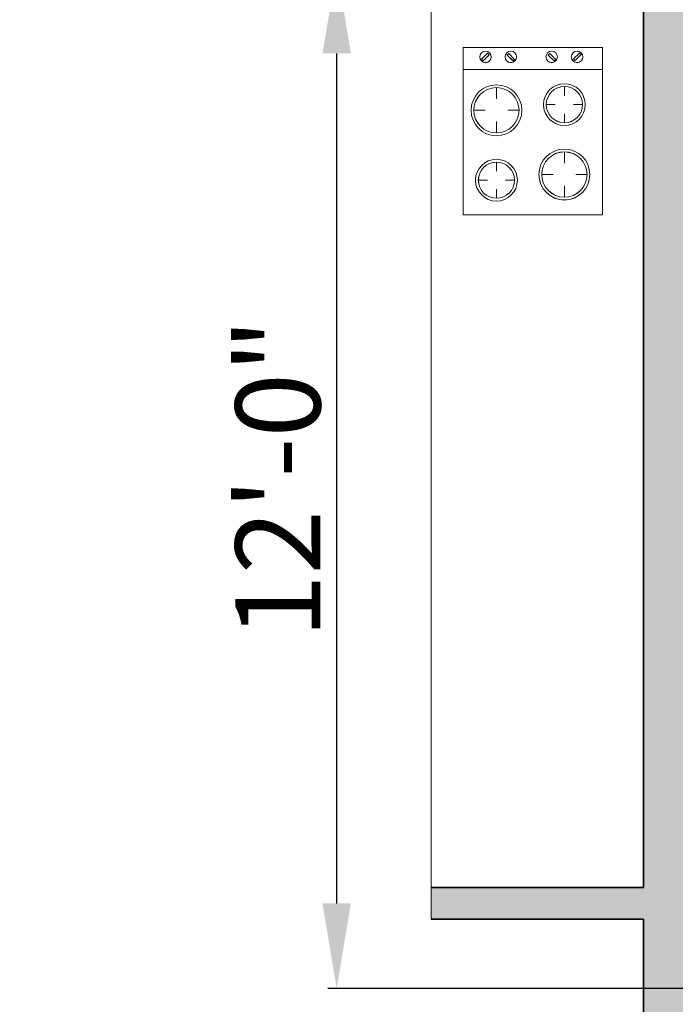
# Model space of a CAD drawing. Units: inches. Extents: x 2083 to 3317, y 1141 to 2115.
# Tile 104 of 256: x 2508 to 2600, y 1794 to 1933. Entities that reach past the tile are written whole.
import ezdxf

# ---------------------------------------------------------------- set-up
doc = ezdxf.new("R2010")
doc.units = ezdxf.units.IN
for name, color, linetype, lineweight in [('A-ANNO-DIMS', 2, 'Continuous', 18), ('A-EQPM', 8, 'Continuous', 18), ('A-FLOR-CASE', 8, 'Continuous', 18), ('A-WALL', 7, 'Continuous', 35)]:
    doc.layers.add(name, color=color, linetype=linetype, lineweight=lineweight)
doc.layers.add('A-WALL-PATT', color=251, linetype='Continuous', lineweight=13, true_color=0x636466)
doc.styles.get("Standard").update_dxf_attribs({"font": 'arial.ttf'})
doc.dimstyles.new('ISO-25', dxfattribs={"dimtxt": 12, "dimasz": 12, "dimexe": 1.25, "dimexo": 0.625, "dimtad": 1, "dimlunit": 3, "dimtxsty": 'Standard', "dimcen": 2.5, "dimadec": 0, "dimazin": 0, "dimtfac": 1, "dimtmove": 0, "dimatfit": 3, "dimfxl": 1, "dimarcsym": 0})

# ---------------------------------------------------------------- blocks, each defined once
blk = doc.blocks.new('A$C16A60262')
at = {"linetype": 'ByBlock'}
for p, q in [((0, 600), (0, 0)), ((487.7, 600), (0, 600)), ((0, 600), (500, 600)), ((0, 600), (500, 600)), ((500, 600), (500, 0)), ((500, 600), (500, 0)), ((500, 520.4), (0, 520.4)), ((363.3, 459.6), (363.3, 427.1)), ((119.4, 455.6), (119.4, 414.9)), ((298.2, 394.6), (330.7, 394.6)), ((428.3, 394.6), (395.8, 394.6)), ((38.1, 374.3), (78.8, 374.3)), ((200.7, 374.3), (160.1, 374.3)), ((363.3, 329.6), (363.3, 362.1)), ((119.4, 293), (119.4, 333.7)), ((363.3, 225.2), (363.3, 184.6)), ((119.4, 188.6), (119.4, 156.1)), ((282, 143.9), (322.6, 143.9)), ((444.5, 143.9), (403.9, 143.9)), ((54.4, 123.6), (86.9, 123.6)), ((184.4, 123.6), (151.9, 123.6)), ((119.4, 58.6), (119.4, 91.1)), ((363.3, 62.6), (363.3, 103.3)), ((0, 0), (500, 0))]:
    blk.add_line(p, q, dxfattribs=at)
for p, q in [((66.2, 557.5), (87.4, 578.7)), ((93.1, 573), (71.9, 551.8)), ((87.4, 578.7), (93.1, 573)), ((157.6, 572.5), (163.3, 578.1)), ((178.8, 551.2), (157.6, 572.5)), ((163.3, 578.1), (184.5, 556.9)), ((305.1, 572.5), (310.8, 578.1)), ((326.3, 551.2), (305.1, 572.5)), ((310.8, 578.1), (332, 556.9)), ((396.2, 558.5), (417.4, 579.7)), ((423.1, 574), (401.9, 552.8)), ((417.4, 579.7), (423.1, 574)), ((71.9, 551.8), (66.2, 557.5)), ((184.5, 556.9), (178.8, 551.2)), ((332, 556.9), (326.3, 551.2)), ((401.9, 552.8), (396.2, 558.5))]:
    blk.add_line(p, q)
for centre in [(80.1, 565.7), (171.2, 565.7), (317.6, 565.7), (408.7, 565.7)]:
    blk.add_circle(centre, 20.6)
for centre, radius in [((119.4, 374.3), 91.3), ((363.3, 394.6), 75), ((363.3, 394.6), 65), ((119.4, 374.3), 81.3), ((363.3, 143.9), 91.3), ((363.3, 143.9), 81.3), ((119.4, 123.6), 75), ((119.4, 123.6), 65)]:
    blk.add_circle(centre, radius, dxfattribs=at)
blk = doc.blocks.new('*D50')
at = {"layer": 'A-ANNO-DIMS', "color": 0, "lineweight": -2, "transparency": 16777216}
for p, q in [((2604.33, 1939.76), (2551.36, 1939.76)), ((2552.61, 1807.76), (2552.61, 1927.76)), ((2604.33, 1795.76), (2551.36, 1795.76))]:
    blk.add_line(p, q, dxfattribs=at)
at = {"layer": 'A-ANNO-DIMS', "color": 0, "transparency": 16777216}
for points in [[(2550.61, 1927.76), (2554.61, 1927.76), (2552.61, 1939.76)], [(2550.61, 1807.76), (2554.61, 1807.76), (2552.61, 1795.76)]]:
    blk.add_solid(points, dxfattribs=at)
at = {"layer": 'Defpoints', "color": 0, "transparency": 16777216}
for p in [(2552.61, 1939.76), (2604.96, 1939.76), (2604.96, 1795.76)]:
    blk.add_point(p, dxfattribs=at)
at = {"layer": 'A-ANNO-DIMS', "color": 0, "transparency": 16777216, "insert": (2545.86, 1867.76), "char_height": 12, "attachment_point": 5, "rotation": 90}
blk.add_mtext('12\'-0"', dxfattribs=at)

msp = doc.modelspace()

# ---------------------------------------------------------------- hatches: boundary and pattern name
at = {"layer": 'A-WALL-PATT'}
h = msp.add_hatch(color=256, dxfattribs=at)
h.dxf.hatch_style = 1
h.paths.add_polyline_path([(3126.96, 2020.761), (2748.96, 2020.761), (2604.96, 2020.761), (2226.96, 2020.761), (2226.96, 1702.761), (2466.96, 1702.761), (2466.96, 1582.761), (2418.96, 1582.761), (2418.96, 1477.761), (2226.96, 1477.761), (2226.96, 1263.261), (2544.96, 1263.261), (2544.96, 1411.761), (2604.96, 1411.761), (2685.96, 1411.761), (2685.96, 1420.761), (2604.96, 1420.761), (2604.96, 1573.761), (2604.96, 1702.761), (2604.96, 2011.761), (2748.96, 2011.761), (2748.96, 1702.761), (2862.96, 1702.761), (2862.96, 1621.761), (2871.96, 1621.761), (2871.96, 1702.761), (2883.96, 1702.761), (2883.96, 1706.939, -0.0264593), (2883.96, 1711.761), (2757.96, 1711.761), (2757.96, 1807.761), (2787.96, 1807.761), (2787.96, 1812.261), (2757.96, 1812.261), (2757.96, 2011.761), (2877.96, 2011.761), (2877.96, 1812.261), (2847.96, 1812.261), (2847.96, 1807.761), (2889.836, 1807.761), (2889.836, 1812.261), (2882.46, 1812.261), (2882.46, 2011.761), (3117.96, 2011.761), (3117.96, 1812.261), (2937.836, 1812.261), (2937.836, 1807.761), (2995.71, 1807.761), (2995.71, 1796.118), (3000.21, 1796.118), (3000.21, 1807.761), (3117.96, 1807.761), (3117.96, 1711.761), (3000.21, 1711.761), (3000.21, 1760.118), (2998.573, 1760.118, -0.020711), (2995.71, 1760.118), (2995.71, 1711.761), (2931.96, 1711.761), (2931.96, 1702.761), (3126.96, 1702.761)])
h.paths.add_polyline_path([(2471.46, 2011.761), (2471.46, 1810.011), (2462.717, 1810.011), (2462.717, 1805.511), (2505.96, 1805.511), (2505.96, 1810.011), (2475.96, 1810.011), (2475.96, 2011.761), (2595.96, 2011.761), (2595.96, 1810.011), (2565.96, 1810.011), (2565.96, 1805.511), (2595.96, 1805.511), (2595.96, 1711.761), (2235.96, 1711.761), (2235.96, 1805.511), (2353.71, 1805.511), (2353.71, 1796.054), (2358.21, 1796.054), (2358.21, 1805.511), (2414.717, 1805.511), (2414.717, 1810.011), (2235.96, 1810.011), (2235.96, 2011.761)], flags=16)
h.paths.add_polyline_path([(2270.205, 1994.61), (2270.205, 1970.61), (2246.205, 1970.61), (2246.205, 1994.61)], flags=0)
edge = h.paths.add_edge_path(flags=0)
edge.add_ellipse((2332.027, 1899.798), major_axis=(-3.043, 3.043), ratio=0.1682525, start_angle=-161.33217, end_angle=-156.30711, ccw=False)
edge.add_ellipse((2333.082, 1898.744), major_axis=(-1.055, 1.055), ratio=0.4535321, start_angle=-123.37102, end_angle=-94.15911)
edge = h.paths.add_edge_path(flags=0)
edge.add_ellipse((2332.027, 1968.876), major_axis=(3.043, 3.043), ratio=0.1682525, start_angle=18.66783, end_angle=23.69289)
edge.add_spline(control_points=[(2332.926, 1970.691), (2332.227, 1970.336), (2330.894, 1969.659), (2328.413, 1970.932), (2327.204, 1967.749), (2324.71, 1969.956), (2322.533, 1967.012), (2320.013, 1971.296), (2317.68, 1968.158), (2316.041, 1967.102), (2315.427, 1966.81)], knot_values=[0, 0, 0, 0, 2.2670587, 4.3245589, 6.6855835, 8.8786411, 11.121502, 14.300359, 17.7552837, 19.732645, 19.732645, 19.732645, 19.732645], degree=3, periodic=0)
edge.add_ellipse((2332.027, 1968.876), major_axis=(3.043, 3.043), ratio=0.1682525, start_angle=18.66783, end_angle=23.69289, ccw=False)
edge.add_ellipse((2333.082, 1969.931), major_axis=(1.055, 1.055), ratio=0.4535321, start_angle=56.62898, end_angle=85.84089, ccw=False)
edge = h.paths.add_edge_path(flags=0)
edge.add_spline(control_points=[(2296.428, 1967.988), (2293.628, 1965.336), (2287.704, 1959.727), (2299.744, 1949.996), (2294.533, 1935.669), (2290.573, 1920.604), (2293.394, 1909.974), (2296.185, 1904.967)], knot_values=[0.0991853, 0.0991853, 0.0991853, 0.0991853, 0.3453009, 0.6198217, 0.9826526, 1.3860932, 1.8105546, 1.8105546, 1.8105546, 1.8105546], degree=3, periodic=0)
edge.add_spline(control_points=[(2296.185, 1904.967), (2297.384, 1902.619), (2298.001, 1901.949), (2298.553, 1901.468)], knot_values=[0.0062457, 0.0062457, 0.0062457, 0.0062457, 0.0554759, 0.0554759, 0.0554759, 0.0554759], degree=3, periodic=0)
edge.add_spline(control_points=[(2298.553, 1901.468), (2297.259, 1900.923), (2295.225, 1900.232), (2293.06, 1900.614), (2292.101, 1900.788), (2292.09, 1900.791)], knot_values=[0.3128349, 0.3128349, 0.3128349, 0.3128349, 0.4017797, 0.4749867, 0.4759027, 0.4759027, 0.4759027, 0.4759027], degree=3, periodic=0)
edge.add_arc((2292.794, 1904.664), 3.937, 215.4209, 259.69818, ccw=False)
edge.add_spline(control_points=[(2289.585, 1902.382), (2289.477, 1902.535), (2289.368, 1902.688), (2289.261, 1902.841)], knot_values=[0.1028719, 0.1028719, 0.1028719, 0.1028719, 0.1168958, 0.1168958, 0.1168958, 0.1168958], degree=3, periodic=0)
edge.add_spline(control_points=[(2289.261, 1902.841), (2288.687, 1902.55), (2287.64, 1902.02), (2285.881, 1901.874), (2283.853, 1901.504), (2281.72, 1899.711), (2278.467, 1899.493), (2276.157, 1901.883), (2272.259, 1899.804), (2267.778, 1901.843), (2262.244, 1900.184), (2257.415, 1901.782), (2254.318, 1900.726), (2253.178, 1900.337)], knot_values=[0, 0, 0, 0, 1.9079767, 3.4771759, 5.261074, 7.9728515, 11.6802485, 13.7179214, 16.9395917, 22.789562, 27.5025027, 33.5952153, 37.1456181, 37.1456181, 37.1456181, 37.1456181], degree=3, periodic=0)
edge.add_line((2253.178, 1900.337), (2250.244, 1902.841))
edge.add_line((2250.244, 1902.841), (2250.244, 1965.833))
edge.add_line((2250.244, 1965.833), (2253.178, 1968.337))
edge.add_spline(control_points=[(2253.178, 1968.337), (2254.318, 1967.948), (2257.415, 1966.892), (2262.244, 1968.49), (2267.778, 1966.831), (2271.527, 1968.537), (2273.876, 1967.828), (2274.207, 1967.728)], knot_values=[0, 0, 0, 0, 0.0901802, 0.2449351, 0.3646438, 0.5132331, 0.5378548, 0.5378548, 0.5378548, 0.5378548], degree=3, periodic=0)
edge.add_arc((2274.353, 1963.793), 3.937, 72.05113, 92.12795, ccw=False)
edge.add_arc((2281.297, 1985.23), 18.596, 252.05113, 288.56572)
edge.add_arc((2292.317, 1956.029), 12.646, 71.02679, 113.77822, ccw=False)
edge = h.paths.add_edge_path(flags=0)
edge.add_spline(control_points=[(2274.899, 1951.856), (2275.066, 1951.617), (2275.233, 1951.377), (2275.398, 1951.136)], knot_values=[1.4099157, 1.4099157, 1.4099157, 1.4099157, 1.4315903, 1.4315903, 1.4315903, 1.4315903], degree=3, periodic=0)
edge.add_spline(control_points=[(2275.398, 1951.136), (2275.792, 1950.562), (2276.179, 1949.984), (2276.546, 1949.397)], knot_values=[1.3582378, 1.3582378, 1.3582378, 1.3582378, 1.4099157, 1.4099157, 1.4099157, 1.4099157], degree=3, periodic=0)
edge.add_line((2276.546, 1949.397), (2277.437, 1947.862))
edge.add_spline(control_points=[(2277.437, 1947.862), (2276.304, 1945.673), (2274.64, 1942.427), (2274.632, 1938.094), (2272.799, 1930.852), (2274.356, 1943.897), (2275.948, 1947.923), (2276.546, 1949.397)], knot_values=[0.0056315, 0.0056315, 0.0056315, 0.0056315, 0.1860139, 0.2660015, 0.3570872, 0.5963902, 0.7397317, 0.7397317, 0.7397317, 0.7397317], degree=3, periodic=0)
edge.add_spline(control_points=[(2276.546, 1949.397), (2276.179, 1949.984), (2275.792, 1950.562), (2275.398, 1951.136)], knot_values=[1.3582378, 1.3582378, 1.3582378, 1.3582378, 1.4099157, 1.4099157, 1.4099157, 1.4099157], degree=3, periodic=0)
edge.add_spline(control_points=[(2275.398, 1951.136), (2274.943, 1950.08), (2274.208, 1948.025), (2273.935, 1944.851), (2272.469, 1937.627), (2273.466, 1945.696), (2274.701, 1951.059), (2274.899, 1951.856)], knot_values=[0.1043639, 0.1043639, 0.1043639, 0.1043639, 0.1896363, 0.2696239, 0.3607096, 0.6000126, 0.6446217, 0.6446217, 0.6446217, 0.6446217], degree=3, periodic=0)
h.paths.add_polyline_path([(2269.168, 1963.128, -0.3575267), (2268.171, 1960.976, -0.0925607), (2268.171, 1939.436, -0.3575267), (2269.168, 1937.285, -0.3575267), (2267.016, 1938.282, -0.1647847), (2254.686, 1938.282, -0.3575267), (2252.534, 1937.285, -0.3575267), (2253.531, 1939.436, -0.0925607), (2253.531, 1960.976, -0.3575267), (2252.534, 1963.128, -0.3575267), (2254.686, 1962.131, -0.1647847), (2267.016, 1962.131, -0.3575267)], flags=0)
h.paths.add_polyline_path([(2248.874, 1967.802), (2248.874, 1957.028), (2249.458, 1957.028), (2249.458, 1911.647), (2248.874, 1911.647), (2248.874, 1900.873), (2246.512, 1900.873, 0.1973271), (2244.15, 1902.457), (2244.15, 1966.218, 0.1973271), (2246.512, 1967.802)], flags=0)
h.paths.add_polyline_path([(2269.168, 1931.389, -0.3575267), (2268.171, 1929.238, -0.0925607), (2268.171, 1907.698, -0.3575267), (2269.168, 1905.547, -0.3575267), (2267.016, 1906.544, -0.1647847), (2254.686, 1906.544, -0.3575267), (2252.534, 1905.547, -0.3575267), (2253.531, 1907.698, -0.0925607), (2253.531, 1929.238, -0.3575267), (2252.534, 1931.389, -0.3575267), (2254.686, 1930.392, -0.1647847), (2267.016, 1930.392, -0.3575267)], flags=0)
edge = h.paths.add_edge_path(flags=0)
edge.add_spline(control_points=[(2276.197, 1906.724), (2276.168, 1909.029), (2276.114, 1913.372), (2270.598, 1924.925), (2273.905, 1919.013), (2275.922, 1916.262), (2275.475, 1912.402), (2277.258, 1910.381), (2276.696, 1908.225), (2276.646, 1906.813), (2276.618, 1906.008)], knot_values=[0, 0, 0, 0, 8.6102597, 16.2212739, 18.8430575, 23.8048978, 27.4408283, 29.3561016, 31.2034776, 33.6506866, 33.6506866, 33.6506866, 33.6506866], degree=3, periodic=0)
edge.add_spline(control_points=[(2276.618, 1906.008), (2276.623, 1905.624), (2276.498, 1904.629), (2275.442, 1903.855), (2274.937, 1903.08), (2274.859, 1902.841)], knot_values=[0.1564884, 0.1564884, 0.1564884, 0.1564884, 0.1843975, 0.2313765, 0.2505985, 0.2505985, 0.2505985, 0.2505985], degree=3, periodic=0)
edge.add_line((2274.859, 1902.841), (2276.506, 1902.841))
edge.add_spline(control_points=[(2276.506, 1902.841), (2276.788, 1903.085), (2277.665, 1904.125), (2278.25, 1904.341), (2277.654, 1908.527), (2278.156, 1906.228), (2278.1, 1905.286), (2278.847, 1904.069), (2277.857, 1903.415), (2277.874, 1902.991), (2277.904, 1902.841)], knot_values=[0.0595743, 0.0595743, 0.0595743, 0.0595743, 0.0807529, 0.1037415, 0.1697201, 0.1760361, 0.2071372, 0.2404744, 0.2623409, 0.2736605, 0.2736605, 0.2736605, 0.2736605], degree=3, periodic=0)
edge.add_line((2277.904, 1902.841), (2280.03, 1902.841))
edge.add_spline(control_points=[(2280.03, 1902.841), (2279.888, 1903.088), (2279.499, 1903.982), (2280.152, 1905.939), (2278.104, 1909.658), (2279.762, 1907.185), (2280.328, 1904.875), (2280.485, 1903.49), (2281.463, 1903.249), (2281.758, 1902.936), (2281.834, 1902.841)], knot_values=[0.013856, 0.013856, 0.013856, 0.013856, 0.0348738, 0.0888667, 0.1078792, 0.1267378, 0.158714, 0.1937575, 0.2174868, 0.2267221, 0.2267221, 0.2267221, 0.2267221], degree=3, periodic=0)
edge.add_spline(control_points=[(2281.834, 1902.841), (2281.788, 1902.827), (2281.647, 1902.783), (2281.396, 1902.859), (2281.088, 1902.985), (2280.721, 1903.061), (2280.333, 1903.026), (2280.125, 1902.899), (2280.03, 1902.841)], knot_values=[0, 0, 0, 0, 0.1441304, 0.435517, 0.7492759, 1.1530457, 1.5483707, 1.878348, 1.878348, 1.878348, 1.878348], degree=3, periodic=0)
edge.add_line((2280.03, 1902.841), (2277.904, 1902.841))
edge.add_spline(control_points=[(2277.904, 1902.841), (2277.893, 1902.796), (2277.865, 1902.68), (2277.607, 1902.687), (2277.274, 1902.801), (2276.838, 1902.62), (2276.584, 1902.789), (2276.506, 1902.841)], knot_values=[0, 0, 0, 0, 0.1271885, 0.3261988, 0.6280094, 1.2435704, 1.5153306, 1.5153306, 1.5153306, 1.5153306], degree=3, periodic=0)
edge.add_line((2276.506, 1902.841), (2274.859, 1902.841))
edge.add_spline(control_points=[(2274.859, 1902.841), (2274.814, 1902.899), (2274.725, 1903.013), (2274.493, 1903.119), (2274.244, 1902.961), (2273.937, 1903.185), (2273.614, 1902.983), (2273.408, 1902.883), (2273.322, 1902.841)], knot_values=[0, 0, 0, 0, 0.2184302, 0.4369566, 0.6879766, 0.9903786, 1.3983955, 1.6918498, 1.6918498, 1.6918498, 1.6918498], degree=3, periodic=0)
edge.add_spline(control_points=[(2273.322, 1902.841), (2273.617, 1903.446), (2274.274, 1904.538), (2276.027, 1904.574), (2276.207, 1906.584), (2276.197, 1906.724)], knot_values=[0.0122268, 0.0122268, 0.0122268, 0.0122268, 0.0594721, 0.1062177, 0.134458, 0.134458, 0.134458, 0.134458], degree=3, periodic=0)
h.paths.add_polyline_path([(2270.776, 1897.79), (2270.776, 1873.79), (2246.776, 1873.79), (2246.776, 1897.79)], flags=0)
h.paths.add_polyline_path([(2353.71, 1760.005), (2353.71, 1760.054), (2358.21, 1760.054, -0.033729)], flags=0)
h.paths.add_polyline_path([(2321.819, 1737.529), (2341.995, 1737.529, -0.4142136), (2343.203, 1736.321), (2343.203, 1721.021, -0.4142136), (2341.995, 1719.813), (2321.819, 1719.813, -0.4142136), (2320.611, 1721.021), (2320.611, 1736.321, -0.4142136)], flags=0)
h.paths.add_polyline_path([(2324.235, 1736.321), (2339.579, 1736.321, -0.4142136), (2341.995, 1733.905), (2341.995, 1725.45, -0.4142136), (2339.579, 1723.034), (2333.681, 1723.034), (2333.845, 1722.045, -0.8706461), (2335.425, 1721.826, -0.767327), (2333.923, 1721.423), (2331.291, 1721.423, -0.767327), (2329.788, 1721.826, -0.8706461), (2331.368, 1722.045), (2331.533, 1723.034), (2324.235, 1723.034, -0.4142136), (2321.819, 1725.45), (2321.819, 1733.905, -0.4142136)], flags=0)
h.paths.add_polyline_path([(2570.484, 1928.615), (2589.684, 1928.615), (2590.169, 1928.615), (2590.169, 1904.993), (2570.484, 1904.993)], flags=0)
h.paths.add_polyline_path([(2574.447, 1927.264, -1), (2572.829, 1927.264, -1)], flags=0)
h.paths.add_polyline_path([(2573.09, 1926.941), (2573.925, 1927.776), (2574.148, 1927.553), (2573.313, 1926.718)], flags=0)
h.paths.add_polyline_path([(2578.779, 1919.73, -1), (2571.592, 1919.73, -1)], flags=0)
h.paths.add_polyline_path([(2578.385, 1919.73, -1), (2571.985, 1919.73, -1)], flags=0)
h.paths.add_polyline_path([(2331.596, 1729.476, -1), (2333.618, 1729.476, -1)], flags=0)
h.paths.add_polyline_path([(2578.034, 1927.264, -1), (2576.416, 1927.264, -1)], flags=0)
h.paths.add_polyline_path([(2576.689, 1927.531), (2576.912, 1927.754), (2577.747, 1926.919), (2577.524, 1926.696)], flags=0)
h.paths.add_polyline_path([(2578.139, 1909.86, -1), (2572.232, 1909.86, -1)], flags=0)
h.paths.add_polyline_path([(2577.745, 1909.86, -1), (2572.625, 1909.86, -1)], flags=0)
h.paths.add_polyline_path([(2583.798, 1927.264, -1), (2582.179, 1927.264, -1)], flags=0)
h.paths.add_polyline_path([(2582.719, 1927.754), (2583.554, 1926.919), (2583.331, 1926.696), (2582.496, 1927.531)], flags=0)
h.paths.add_polyline_path([(2582.496, 1927.531), (2582.719, 1927.754), (2583.554, 1926.919), (2583.331, 1926.696)], flags=0)
h.paths.add_polyline_path([(2587.739, 1920.53, -1), (2581.832, 1920.53, -1)], flags=0)
h.paths.add_polyline_path([(2587.345, 1920.53, -1), (2582.225, 1920.53, -1)], flags=0)
h.paths.add_polyline_path([(2587.385, 1927.264, -1), (2585.766, 1927.264, -1)], flags=0)
h.paths.add_polyline_path([(2586.082, 1926.98), (2586.917, 1927.815), (2587.14, 1927.593), (2586.305, 1926.758)], flags=0)
h.paths.add_polyline_path([(2588.379, 1910.66, -1), (2581.192, 1910.66, -1)], flags=0)
h.paths.add_polyline_path([(2587.985, 1910.66, -1), (2581.585, 1910.66, -1)], flags=0)
h.paths.add_polyline_path([(2417.168, 1729.478), (2437.344, 1729.478, -0.4142136), (2438.552, 1728.27), (2438.552, 1712.969, -0.4142136), (2437.344, 1711.761), (2417.168, 1711.761, -0.4142136), (2415.96, 1712.969), (2415.96, 1728.27, -0.4142136)], flags=0)
h.paths.add_polyline_path([(2419.584, 1728.27), (2434.928, 1728.27, -0.4142136), (2437.344, 1725.854), (2437.344, 1717.398, -0.4142136), (2434.928, 1714.983), (2429.029, 1714.983), (2429.194, 1713.994, -0.8706461), (2430.774, 1713.775, -0.767327), (2429.271, 1713.372), (2426.64, 1713.372, -0.767327), (2425.137, 1713.775, -0.8706461), (2426.717, 1713.994), (2426.882, 1714.983), (2419.584, 1714.983, -0.4142136), (2417.168, 1717.398), (2417.168, 1725.854, -0.4142136)], flags=0)
h.paths.add_polyline_path([(2419.584, 1728.27), (2434.928, 1728.27, -0.4142136), (2437.344, 1725.854), (2437.344, 1717.398, -0.4142136), (2434.928, 1714.983), (2429.029, 1714.983), (2428.358, 1719.009), (2427.553, 1719.009), (2426.882, 1714.983), (2419.584, 1714.983, -0.4142136), (2417.168, 1717.398), (2417.168, 1725.854, -0.4142136)], flags=0)
h.paths.add_polyline_path([(2426.944, 1721.425, -1), (2428.967, 1721.425, -1)], flags=0)
h.paths.add_polyline_path([(2475.96, 1702.761), (2595.96, 1702.761), (2595.96, 1582.761), (2475.96, 1582.761)], flags=16)
h.paths.add_polyline_path([(2427.96, 1573.761), (2595.96, 1573.761), (2595.96, 1468.761), (2595.96, 1420.761), (2384.46, 1420.761), (2384.46, 1468.761), (2427.96, 1468.761)], flags=16)
h.paths.add_polyline_path([(2379.96, 1468.761), (2379.96, 1420.761), (2235.96, 1420.761), (2235.96, 1468.761)], flags=16)
h.paths.add_polyline_path([(2317.816, 1466.696), (2337.992, 1466.696, -0.4142136), (2339.2, 1465.488), (2339.2, 1450.187, -0.4142136), (2337.992, 1448.979), (2317.816, 1448.979, -0.4142136), (2316.608, 1450.187), (2316.608, 1465.488, -0.4142136)], flags=0)
h.paths.add_polyline_path([(2320.232, 1465.488), (2335.576, 1465.488, -0.4142136), (2337.992, 1463.072), (2337.992, 1454.616, -0.4142136), (2335.576, 1452.2), (2329.677, 1452.2), (2329.842, 1451.212, -0.8706461), (2331.422, 1450.992, -0.767327), (2329.92, 1450.59), (2327.288, 1450.59, -0.767327), (2325.785, 1450.992, -0.8706461), (2327.365, 1451.212), (2327.53, 1452.2), (2320.232, 1452.2, -0.4142136), (2317.816, 1454.616), (2317.816, 1463.072, -0.4142136)], flags=0)
h.paths.add_polyline_path([(2320.232, 1465.488), (2335.576, 1465.488, -0.4142136), (2337.992, 1463.072), (2337.992, 1454.616, -0.4142136), (2335.576, 1452.2), (2329.677, 1452.2), (2329.006, 1456.227), (2328.201, 1456.227), (2327.53, 1452.2), (2320.232, 1452.2, -0.4142136), (2317.816, 1454.616), (2317.816, 1463.072, -0.4142136)], flags=0)
h.paths.add_polyline_path([(2327.593, 1458.643, -1), (2329.615, 1458.643, -1)], flags=0)
h.paths.add_polyline_path([(2244.412, 1433.34), (2241.921, 1433.34, -0.4142136), (2240.018, 1435.244), (2240.018, 1440.953, -0.4142105), (2241.921, 1442.856), (2244.412, 1442.856, -1.9764724)], flags=0)
h.paths.add_polyline_path([(2245.357, 1434.398, -0.4142136), (2245.357, 1441.799, -2.1440985)], flags=0)
h.paths.add_polyline_path([(2535.96, 1416.261), (2535.96, 1272.261), (2235.96, 1272.261), (2235.96, 1416.261)], flags=16)
h.paths.add_polyline_path([(2260.12, 1384.293), (2260.12, 1362.039), (2237.865, 1362.039), (2237.865, 1384.293)], flags=0)
edge = h.paths.add_edge_path(flags=0)
edge.add_line((2318.252, 1362.093), (2318.146, 1362.001))
edge.add_ellipse((2317.445, 1360.431), major_axis=(2.822, 2.822), ratio=0.1682525, start_angle=18.66783, end_angle=20.94813, ccw=False)
edge.add_ellipse((2318.423, 1361.409), major_axis=(0.978, 0.978), ratio=0.4535321, start_angle=56.62898, end_angle=70.2262, ccw=False)
edge = h.paths.add_edge_path(flags=0)
edge.add_line((2319.107, 1295.571), (2319.015, 1295.677))
edge.add_ellipse((2317.445, 1296.378), major_axis=(-2.822, 2.822), ratio=0.1682525, start_angle=-161.33217, end_angle=-159.05187, ccw=False)
edge.add_ellipse((2318.423, 1295.4), major_axis=(-0.978, 0.978), ratio=0.4535321, start_angle=-123.37102, end_angle=-109.7738)
edge = h.paths.add_edge_path(flags=0)
edge.add_spline(control_points=[(2284.21, 1301.17), (2284.581, 1300.445), (2284.891, 1299.892), (2285.16, 1299.461)], knot_values=[0.0390658, 0.0390658, 0.0390658, 0.0390658, 0.0554759, 0.0554759, 0.0554759, 0.0554759], degree=3, periodic=0)
edge.add_line((2285.16, 1299.461), (2284.21, 1301.17))
edge = h.paths.add_edge_path(flags=0)
edge.add_line((2280.412, 1297.298), (2283.37, 1297.036))
edge.add_line((2283.37, 1297.036), (2286.406, 1297.926))
edge.add_spline(control_points=[(2286.406, 1297.926), (2285.305, 1297.463), (2284.345, 1297.129), (2283.37, 1297.036)], knot_values=[0.3943688, 0.3943688, 0.3943688, 0.3943688, 0.4759027, 0.4759027, 0.4759027, 0.4759027], degree=3, periodic=0)
edge.add_spline(control_points=[(2283.37, 1297.036), (2283.281, 1297.028), (2282.316, 1296.957), (2281.313, 1297.134), (2280.423, 1297.296), (2280.412, 1297.298)], knot_values=[0.3128349, 0.3128349, 0.3128349, 0.3128349, 0.3202458, 0.3934528, 0.3943688, 0.3943688, 0.3943688, 0.3943688], degree=3, periodic=0)
edge = h.paths.add_edge_path(flags=0)
edge.add_line((2284.436, 1359.607), (2280.446, 1355.328))
edge.add_line((2280.446, 1355.328), (2279.58, 1351.018))
edge.add_line((2279.58, 1351.018), (2282.413, 1346.58))
edge.add_spline(control_points=[(2282.413, 1346.58), (2283.153, 1345.589), (2284.253, 1344.029), (2284.801, 1342.387), (2284.935, 1341.806)], knot_values=[1.2400982, 1.2400982, 1.2400982, 1.2400982, 1.3328922, 1.3827123, 1.3827123, 1.3827123, 1.3827123], degree=3, periodic=0)
edge.add_spline(control_points=[(2284.935, 1341.806), (2285.319, 1340.141), (2285.233, 1338.409), (2284.91, 1336.654)], knot_values=[1.0974841, 1.0974841, 1.0974841, 1.0974841, 1.2400982, 1.2400982, 1.2400982, 1.2400982], degree=3, periodic=0)
edge.add_spline(control_points=[(2284.91, 1336.654), (2284.587, 1334.899), (2284.027, 1333.12), (2283.463, 1331.361)], knot_values=[0.9548699, 0.9548699, 0.9548699, 0.9548699, 1.0974841, 1.0974841, 1.0974841, 1.0974841], degree=3, periodic=0)
edge.add_line((2283.463, 1331.361), (2281.89, 1326.153))
edge.add_line((2281.89, 1326.153), (2280.756, 1321.056))
edge.add_line((2280.756, 1321.056), (2280.299, 1316.002))
edge.add_line((2280.299, 1316.002), (2280.716, 1310.95))
edge.add_line((2280.716, 1310.95), (2282.028, 1305.972))
edge.add_line((2282.028, 1305.972), (2284.21, 1301.17))
edge.add_spline(control_points=[(2284.21, 1301.17), (2283.341, 1302.73), (2282.612, 1304.336), (2282.028, 1305.972)], knot_values=[0.0991853, 0.0991853, 0.0991853, 0.0991853, 0.2417994, 0.2417994, 0.2417994, 0.2417994], degree=3, periodic=0)
edge.add_spline(control_points=[(2282.028, 1305.972), (2281.444, 1307.608), (2281.005, 1309.273), (2280.716, 1310.95)], knot_values=[0.2417994, 0.2417994, 0.2417994, 0.2417994, 0.3844135, 0.3844135, 0.3844135, 0.3844135], degree=3, periodic=0)
edge.add_spline(control_points=[(2280.716, 1310.95), (2280.433, 1312.588), (2280.289, 1314.277), (2280.299, 1315.962), (2280.299, 1316.002)], knot_values=[0.3844135, 0.3844135, 0.3844135, 0.3844135, 0.5236467, 0.5270276, 0.5270276, 0.5270276, 0.5270276], degree=3, periodic=0)
edge.add_spline(control_points=[(2280.299, 1316.002), (2280.312, 1317.687), (2280.478, 1319.368), (2280.756, 1321.056)], knot_values=[0.5270276, 0.5270276, 0.5270276, 0.5270276, 0.6696417, 0.6696417, 0.6696417, 0.6696417], degree=3, periodic=0)
edge.add_spline(control_points=[(2280.756, 1321.056), (2281.035, 1322.744), (2281.426, 1324.44), (2281.89, 1326.153)], knot_values=[0.6696417, 0.6696417, 0.6696417, 0.6696417, 0.8122558, 0.8122558, 0.8122558, 0.8122558], degree=3, periodic=0)
edge.add_spline(control_points=[(2281.89, 1326.153), (2282.264, 1327.533), (2282.788, 1329.262), (2283.353, 1331.018), (2283.463, 1331.361)], knot_values=[0.8122558, 0.8122558, 0.8122558, 0.8122558, 0.9270873, 0.9548699, 0.9548699, 0.9548699, 0.9548699], degree=3, periodic=0)
edge.add_line((2283.463, 1331.361), (2284.91, 1336.654))
edge.add_line((2284.91, 1336.654), (2284.935, 1341.806))
edge.add_line((2284.935, 1341.806), (2282.413, 1346.58))
edge.add_spline(control_points=[(2282.413, 1346.58), (2281.275, 1348.104), (2280.078, 1349.57), (2279.58, 1351.018)], knot_values=[1.3827123, 1.3827123, 1.3827123, 1.3827123, 1.5253264, 1.5253264, 1.5253264, 1.5253264], degree=3, periodic=0)
edge.add_spline(control_points=[(2279.58, 1351.018), (2279.443, 1351.415), (2279.136, 1352.857), (2279.735, 1354.29), (2280.446, 1355.328)], knot_values=[1.5253264, 1.5253264, 1.5253264, 1.5253264, 1.564439, 1.6679405, 1.6679405, 1.6679405, 1.6679405], degree=3, periodic=0)
edge.add_spline(control_points=[(2280.446, 1355.328), (2281.426, 1356.758), (2282.931, 1358.183), (2284.436, 1359.607)], knot_values=[1.6679405, 1.6679405, 1.6679405, 1.6679405, 1.8105546, 1.8105546, 1.8105546, 1.8105546], degree=3, periodic=0)
edge.add_arc((2280.623, 1348.518), 11.726, 71.02679, 113.77822)
edge.add_arc((2270.405, 1375.595), 17.244, 252.05113, 288.56572, ccw=False)
edge.add_arc((2263.966, 1355.718), 3.651, 72.05113, 92.12795)
edge.add_arc((2263.966, 1355.718), 3.651, 92.12795, 177.98513)
edge.add_spline(control_points=[(2260.318, 1355.846), (2260.26, 1354.221), (2260.551, 1350.187), (2262.999, 1346.766), (2264.473, 1344.649)], knot_values=[1.4315903, 1.4315903, 1.4315903, 1.4315903, 1.5641438, 1.7706953, 1.7706953, 1.7706953, 1.7706953], degree=3, periodic=0)
edge.add_line((2264.473, 1344.649), (2264.936, 1343.983))
edge.add_spline(control_points=[(2263.801, 1340.248), (2263.843, 1340.514), (2264.067, 1341.756), (2264.513, 1343.002), (2264.935, 1343.981)], knot_values=[0.5365702, 0.5365702, 0.5365702, 0.5365702, 0.5593494, 0.6446217, 0.6446217, 0.6446217, 0.6446217], degree=3, periodic=0)
edge.add_spline(control_points=[(2264.935, 1343.981), (2265.118, 1343.715), (2265.299, 1343.448), (2265.477, 1343.179)], knot_values=[1.3840767, 1.3840767, 1.3840767, 1.3840767, 1.4099157, 1.4099157, 1.4099157, 1.4099157], degree=3, periodic=0)
edge.add_spline(control_points=[(2265.477, 1343.179), (2265.655, 1342.911), (2265.829, 1342.641), (2265.999, 1342.369)], knot_values=[1.3582378, 1.3582378, 1.3582378, 1.3582378, 1.3840767, 1.3840767, 1.3840767, 1.3840767], degree=3, periodic=0)
edge.add_line((2265.999, 1342.369), (2266.826, 1340.946))
edge.add_spline(control_points=[(2266.826, 1340.946), (2268.894, 1337.09), (2271.398, 1325.843), (2270.516, 1310.569), (2275.919, 1301.861), (2277.79, 1299.199)], knot_values=[0.1168958, 0.1168958, 0.1168958, 0.1168958, 0.4729873, 1.0509689, 1.3137934, 1.3137934, 1.3137934, 1.3137934], degree=3, periodic=0)
edge.add_spline(control_points=[(2277.79, 1299.199), (2277.839, 1299.128), (2277.889, 1299.057), (2277.94, 1298.987)], knot_values=[0.1098839, 0.1098839, 0.1098839, 0.1098839, 0.1168958, 0.1168958, 0.1168958, 0.1168958], degree=3, periodic=0)
edge.add_line((2277.94, 1298.987), (2277.789, 1299.199))
edge.add_spline(control_points=[(2277.789, 1299.199), (2277.257, 1298.929), (2276.286, 1298.438), (2275.039, 1298.334), (2274.383, 1298.239), (2274.215, 1298.209)], knot_values=[33.1218702, 33.1218702, 33.1218702, 33.1218702, 35.0290557, 36.5982549, 37.1448269, 37.1448269, 37.1448269, 37.1448269], degree=3, periodic=0)
edge.add_line((2274.215, 1298.209), (2273.073, 1297.893))
edge.add_spline(control_points=[(2273.073, 1297.893), (2272.323, 1297.58), (2271.039, 1296.511), (2269.248, 1296.226), (2268.423, 1296.375)], knot_values=[26.5325843, 26.5325843, 26.5325843, 26.5325843, 29.198919, 31.8391012, 31.8391012, 31.8391012, 31.8391012], degree=3, periodic=0)
edge.add_line((2268.423, 1296.375), (2263.879, 1297.458))
edge.add_spline(control_points=[(2263.879, 1297.458), (2263.556, 1297.359), (2261.86, 1296.839), (2260.239, 1297.282), (2258.933, 1297.516)], knot_values=[15.9195506, 15.9195506, 15.9195506, 15.9195506, 16.9395917, 21.2260675, 21.2260675, 21.2260675, 21.2260675], degree=3, periodic=0)
edge.add_line((2258.933, 1297.516), (2254.055, 1297.329))
edge.add_spline(control_points=[(2254.055, 1297.329), (2253.756, 1297.296), (2252.114, 1297.165), (2250.462, 1297.544), (2249.13, 1297.668)], knot_values=[5.3065169, 5.3065169, 5.3065169, 5.3065169, 6.2764352, 10.6130337, 10.6130337, 10.6130337, 10.6130337], degree=3, periodic=0)
edge.add_line((2249.13, 1297.668), (2244.332, 1296.878))
edge.add_line((2244.332, 1296.878), (2241.611, 1299.199))
edge.add_line((2241.611, 1299.199), (2241.611, 1357.609))
edge.add_line((2241.611, 1357.609), (2244.332, 1359.931))
edge.add_line((2244.332, 1359.931), (2252.729, 1359.543))
edge.add_spline(control_points=[(2252.729, 1359.543), (2252.871, 1359.546), (2253.306, 1359.548), (2253.74, 1359.514), (2254.032, 1359.482)], knot_values=[0.233291, 0.233291, 0.233291, 0.233291, 0.2449351, 0.2689274, 0.2689274, 0.2689274, 0.2689274], degree=3, periodic=0)
edge.add_line((2254.032, 1359.482), (2259.587, 1359.416))
edge.add_spline(control_points=[(2259.587, 1359.416), (2260.677, 1359.629), (2262.073, 1359.897), (2263.524, 1359.459), (2263.83, 1359.366)], knot_values=[0.4225164, 0.4225164, 0.4225164, 0.4225164, 0.5132331, 0.5378548, 0.5378548, 0.5378548, 0.5378548], degree=3, periodic=0)
edge.add_arc((2263.966, 1355.718), 3.651, 72.05113, 92.12795, ccw=False)
edge.add_arc((2270.405, 1375.595), 17.244, 252.05113, 288.56572)
edge.add_arc((2280.623, 1348.518), 11.726, 71.02679, 113.77822, ccw=False)
h.paths.add_polyline_path([(2240.341, 1359.435), (2240.341, 1349.444), (2240.882, 1349.444), (2240.882, 1307.365), (2240.341, 1307.365), (2240.341, 1297.374), (2238.15, 1297.374, 0.1973271), (2235.96, 1298.843), (2235.96, 1357.966, 0.1973271), (2238.15, 1359.435)], flags=0)
h.paths.add_polyline_path([(2259.158, 1355.101, -0.3575267), (2258.233, 1353.106, -0.0925607), (2258.233, 1333.133, -0.3575267), (2259.158, 1331.138, -0.3575267), (2257.163, 1332.062, -0.1647847), (2245.729, 1332.062, -0.3575267), (2243.735, 1331.138, -0.3575267), (2244.659, 1333.133, -0.0925607), (2244.659, 1353.106, -0.3575267), (2243.735, 1355.101, -0.3575267), (2245.729, 1354.176, -0.1647847), (2257.163, 1354.176, -0.3575267)], flags=0)
edge = h.paths.add_edge_path(flags=0)
edge.add_line((2265.999, 1342.369), (2266.826, 1340.946))
edge.add_line((2266.826, 1340.946), (2265.308, 1337.814))
edge.add_line((2265.308, 1337.814), (2264.358, 1334.653))
edge.add_line((2264.358, 1334.653), (2264.262, 1333.8))
edge.add_spline(control_points=[(2264.262, 1333.8), (2264.208, 1333.187), (2264.162, 1332.366), (2264.007, 1331.414), (2263.969, 1331.202)], knot_values=[0.4644442, 0.4644442, 0.4644442, 0.4644442, 0.5166905, 0.5316081, 0.5316081, 0.5316081, 0.5316081], degree=3, periodic=0)
edge.add_spline(control_points=[(2263.969, 1331.202), (2263.775, 1330.119), (2263.424, 1328.791), (2263.257, 1328.531), (2263.234, 1328.515)], knot_values=[0.3726816, 0.3726816, 0.3726816, 0.3726816, 0.4488497, 0.4644442, 0.4644442, 0.4644442, 0.4644442], degree=3, periodic=0)
edge.add_spline(control_points=[(2263.234, 1328.515), (2263.096, 1328.42), (2263.131, 1329.301), (2263.275, 1330.616)], knot_values=[0.2809191, 0.2809191, 0.2809191, 0.2809191, 0.3726816, 0.3726816, 0.3726816, 0.3726816], degree=3, periodic=0)
edge.add_spline(control_points=[(2263.275, 1330.616), (2263.419, 1331.93), (2263.672, 1333.677), (2263.97, 1335.315)], knot_values=[0.1891566, 0.1891566, 0.1891566, 0.1891566, 0.2809191, 0.2809191, 0.2809191, 0.2809191], degree=3, periodic=0)
edge.add_spline(control_points=[(2263.97, 1335.315), (2264.1, 1336.032), (2264.419, 1337.622), (2264.755, 1338.864), (2264.947, 1339.491)], knot_values=[0.097394, 0.097394, 0.097394, 0.097394, 0.1375775, 0.1891566, 0.1891566, 0.1891566, 0.1891566], degree=3, periodic=0)
edge.add_spline(control_points=[(2264.947, 1339.491), (2265.29, 1340.606), (2265.644, 1341.494), (2265.999, 1342.369)], knot_values=[0.0056315, 0.0056315, 0.0056315, 0.0056315, 0.097394, 0.097394, 0.097394, 0.097394], degree=3, periodic=0)
h.paths.add_polyline_path([(2259.158, 1325.671, -0.3575267), (2258.233, 1323.676, -0.0925607), (2258.233, 1303.703, -0.3575267), (2259.158, 1301.708, -0.3575267), (2257.163, 1302.633, -0.1647847), (2245.729, 1302.633, -0.3575267), (2243.735, 1301.708, -0.3575267), (2244.659, 1303.703, -0.0925607), (2244.659, 1323.676, -0.3575267), (2243.735, 1325.671, -0.3575267), (2245.729, 1324.747, -0.1647847), (2257.163, 1324.747, -0.3575267)], flags=0)
edge = h.paths.add_edge_path(flags=0)
edge.add_spline(control_points=[(2261.709, 1317.311), (2261.679, 1317.418), (2261.762, 1317.389), (2262.491, 1316.09), (2262.962, 1315.301)], knot_values=[14.9558607, 14.9558607, 14.9558607, 14.9558607, 16.2212739, 18.6948259, 18.6948259, 18.6948259, 18.6948259], degree=3, periodic=0)
edge.add_spline(control_points=[(2262.962, 1315.301), (2262.99, 1315.254), (2263.702, 1314.067), (2264.349, 1313.127), (2264.73, 1312.164)], knot_values=[18.6948259, 18.6948259, 18.6948259, 18.6948259, 18.8430575, 22.433791, 22.433791, 22.433791, 22.433791], degree=3, periodic=0)
edge.add_spline(control_points=[(2264.73, 1312.164), (2264.876, 1311.796), (2265.177, 1310.77), (2265.143, 1309.559), (2265.248, 1308.824)], knot_values=[22.433791, 22.433791, 22.433791, 22.433791, 23.8048978, 26.1727562, 26.1727562, 26.1727562, 26.1727562], degree=3, periodic=0)
edge.add_line((2265.248, 1308.824), (2265.851, 1307.172))
edge.add_spline(control_points=[(2265.851, 1307.172), (2266.065, 1306.822), (2266.384, 1306.332), (2266.424, 1305.781), (2266.42, 1305.611)], knot_values=[28.0625624, 28.0625624, 28.0625624, 28.0625624, 29.3561016, 29.9117214, 29.9117214, 29.9117214, 29.9117214], degree=3, periodic=0)
edge.add_spline(control_points=[(2266.42, 1305.611), (2266.416, 1305.433), (2266.394, 1305.25), (2266.365, 1305.066)], knot_values=[29.9117214, 29.9117214, 29.9117214, 29.9117214, 30.4978371, 30.4978371, 30.4978371, 30.4978371], degree=3, periodic=0)
edge.add_line((2266.365, 1305.066), (2266.066, 1302.136))
edge.add_spline(control_points=[(2266.066, 1302.136), (2266.071, 1301.78), (2265.998, 1301.2), (2265.663, 1300.759), (2265.509, 1300.586)], knot_values=[0.1564884, 0.1564884, 0.1564884, 0.1564884, 0.1843975, 0.2035434, 0.2035434, 0.2035434, 0.2035434], degree=3, periodic=0)
edge.add_line((2265.509, 1300.586), (2264.435, 1299.199))
edge.add_line((2264.435, 1299.199), (2265.962, 1299.199))
edge.add_line((2265.962, 1299.199), (2267.336, 1301.175))
edge.add_line((2267.336, 1301.175), (2267.312, 1301.986))
edge.add_spline(control_points=[(2267.312, 1301.986), (2267.261, 1302.862), (2267.16, 1303.737), (2267.271, 1303.326)], knot_values=[0.1262286, 0.1262286, 0.1262286, 0.1262286, 0.1666174, 0.1666174, 0.1666174, 0.1666174], degree=3, periodic=0)
edge.add_spline(control_points=[(2267.271, 1303.326), (2267.28, 1303.294), (2267.31, 1303.175), (2267.373, 1302.884), (2267.406, 1302.683), (2267.418, 1302.601)], knot_values=[0.1666174, 0.1666174, 0.1666174, 0.1666174, 0.1697201, 0.1760361, 0.1807647, 0.1807647, 0.1807647, 0.1807647], degree=3, periodic=0)
edge.add_spline(control_points=[(2267.744, 1300.988), (2267.688, 1301.151), (2267.481, 1301.657), (2267.484, 1302.145), (2267.418, 1302.601)], knot_values=[0.1807647, 0.1807647, 0.1807647, 0.1807647, 0.1937665, 0.2201389, 0.2201389, 0.2201389, 0.2201389], degree=3, periodic=0)
edge.add_line((2267.418, 1302.601), (2267.744, 1300.988))
edge.add_spline(control_points=[(2267.744, 1300.988), (2267.832, 1300.732), (2267.932, 1300.31), (2267.555, 1299.975), (2267.429, 1299.829)], knot_values=[0.2201389, 0.2201389, 0.2201389, 0.2201389, 0.2404744, 0.2548903, 0.2548903, 0.2548903, 0.2548903], degree=3, periodic=0)
edge.add_line((2267.429, 1299.829), (2267.258, 1299.199))
edge.add_line((2267.258, 1299.199), (2269.23, 1299.199))
edge.add_spline(control_points=[(2269.23, 1299.199), (2269.099, 1299.429), (2268.843, 1300.016), (2269.012, 1300.916), (2268.947, 1301.661)], knot_values=[0.013856, 0.013856, 0.013856, 0.013856, 0.0348738, 0.0670726, 0.0670726, 0.0670726, 0.0670726], degree=3, periodic=0)
edge.add_line((2268.947, 1301.661), (2268.432, 1303.603))
edge.add_spline(control_points=[(2268.432, 1303.603), (2268.176, 1304.192), (2267.596, 1305.251), (2268.041, 1304.623), (2268.251, 1304.282)], knot_values=[0.0901547, 0.0901547, 0.0901547, 0.0901547, 0.1078792, 0.1202891, 0.1202891, 0.1202891, 0.1202891], degree=3, periodic=0)
edge.add_spline(control_points=[(2268.251, 1304.282), (2268.361, 1304.105), (2269.058, 1302.918), (2269.383, 1301.59), (2269.521, 1300.776), (2269.575, 1300.556)], knot_values=[0.1202891, 0.1202891, 0.1202891, 0.1202891, 0.1267378, 0.158714, 0.1735056, 0.1735056, 0.1735056, 0.1735056], degree=3, periodic=0)
edge.add_line((2269.575, 1300.556), (2270.686, 1299.421))
edge.add_spline(control_points=[(2270.686, 1299.421), (2270.767, 1299.357), (2270.838, 1299.281), (2270.903, 1299.199)], knot_values=[0.2181597, 0.2181597, 0.2181597, 0.2181597, 0.2267221, 0.2267221, 0.2267221, 0.2267221], degree=3, periodic=0)
edge.add_line((2270.937, 1299.193), (2270.903, 1299.199))
edge.add_spline(control_points=[(2270.903, 1299.199), (2270.86, 1299.186), (2270.73, 1299.146), (2270.496, 1299.216), (2270.272, 1299.308), (2270.121, 1299.348), (2270.063, 1299.36)], knot_values=[0.939174, 0.939174, 0.939174, 0.939174, 1.0833044, 1.3746911, 1.6884499, 1.878348, 1.878348, 1.878348, 1.878348], degree=3, periodic=0)
edge.add_line((2270.063, 1299.36), (2269.23, 1299.199))
edge.add_line((2269.23, 1299.199), (2267.258, 1299.199))
edge.add_spline(control_points=[(2267.258, 1299.199), (2267.248, 1299.157), (2267.223, 1299.05), (2266.984, 1299.057), (2266.809, 1299.116), (2266.677, 1299.109), (2266.637, 1299.105)], knot_values=[0.7576653, 0.7576653, 0.7576653, 0.7576653, 0.8848538, 1.0838641, 1.3856747, 1.5153306, 1.5153306, 1.5153306, 1.5153306], degree=3, periodic=0)
edge.add_spline(control_points=[(2266.637, 1299.105), (2266.485, 1299.089), (2266.236, 1299.017), (2266.035, 1299.151), (2265.962, 1299.199)], knot_values=[0, 0, 0, 0, 0.4859051, 0.7576653, 0.7576653, 0.7576653, 0.7576653], degree=3, periodic=0)
edge.add_line((2265.962, 1299.199), (2264.435, 1299.199))
edge.add_line((2264.435, 1299.199), (2263.858, 1299.367))
edge.add_spline(control_points=[(2263.858, 1299.367), (2263.819, 1299.371), (2263.78, 1299.386), (2263.74, 1299.402)], knot_values=[0.8459249, 0.8459249, 0.8459249, 0.8459249, 0.9786272, 0.9786272, 0.9786272, 0.9786272], degree=3, periodic=0)
edge.add_line((2263.722, 1299.396), (2263.01, 1299.199))
edge.add_spline(control_points=[(2263.01, 1299.199), (2263.246, 1299.683), (2263.506, 1300.128), (2263.873, 1300.408)], knot_values=[0.0122268, 0.0122268, 0.0122268, 0.0122268, 0.0529705, 0.0529705, 0.0529705, 0.0529705], degree=3, periodic=0)
edge.add_spline(control_points=[(2263.873, 1300.408), (2263.932, 1300.453), (2264.084, 1300.553), (2264.255, 1300.624), (2264.36, 1300.665)], knot_values=[0.0529705, 0.0529705, 0.0529705, 0.0529705, 0.0594721, 0.0690861, 0.0690861, 0.0690861, 0.0690861], degree=3, periodic=0)
edge.add_line((2264.36, 1300.665), (2265.142, 1301.078))
edge.add_line((2265.142, 1301.078), (2265.676, 1302.8))
edge.add_line((2265.676, 1302.8), (2265.541, 1305.704))
edge.add_line((2265.541, 1305.704), (2264.803, 1309.328))
edge.add_line((2264.803, 1309.328), (2263.041, 1314.092))
edge.add_spline(control_points=[(2263.041, 1314.092), (2262.384, 1315.671), (2261.796, 1316.998), (2261.709, 1317.311)], knot_values=[11.2168955, 11.2168955, 11.2168955, 11.2168955, 14.9558607, 14.9558607, 14.9558607, 14.9558607], degree=3, periodic=0)
h.paths.add_polyline_path([(2871.96, 1416.261), (2895.91, 1416.261), (2895.91, 1420.761), (2871.96, 1420.761), (2871.96, 1501.761), (2862.96, 1501.761), (2862.96, 1420.761), (2805.96, 1420.761), (2805.96, 1411.761), (2862.96, 1411.761), (2862.96, 1263.261), (3126.96, 1263.261), (3126.96, 1411.761), (3126.96, 1486.761), (2943.96, 1486.761), (2943.96, 1477.761), (2967.86, 1477.761), (2967.86, 1420.761), (2943.91, 1420.761), (2943.91, 1416.261), (3117.96, 1416.261), (3117.96, 1420.761), (2972.36, 1420.761), (2972.36, 1477.761), (3117.96, 1477.761), (3117.96, 1420.761), (3117.96, 1272.261), (2871.96, 1272.261)], flags=0)
h.paths.add_polyline_path([(2457.126, 1485.943), (2527.603, 1485.943), (2527.603, 1537.636), (2457.126, 1537.636)], flags=8)
h.paths.add_polyline_path([(2481.005, 1609.982), (2590.766, 1609.982), (2590.766, 1682.003), (2481.005, 1682.003)], flags=8)
h.paths.add_polyline_path([(2483.085, 1729.127), (2553.562, 1729.127), (2553.562, 1780.82), (2483.085, 1780.82)], flags=8)

# ---------------------------------------------------------------- linework, layer by layer
at = {"layer": 'A-EQPM'}
for p, q in [((2570.484, 1928.615), (2589.684, 1928.615)), ((2570.484, 1904.993), (2570.484, 1928.615)), ((2589.684, 1928.615), (2590.169, 1928.615)), ((2590.169, 1928.615), (2590.169, 1904.993)), ((2573.09, 1926.941), (2573.925, 1927.776)), ((2573.313, 1926.718), (2573.09, 1926.941)), ((2574.148, 1927.553), (2573.313, 1926.718)), ((2573.925, 1927.776), (2574.148, 1927.553)), ((2576.689, 1927.531), (2576.912, 1927.754)), ((2577.524, 1926.696), (2576.689, 1927.531)), ((2576.912, 1927.754), (2577.747, 1926.919)), ((2577.747, 1926.919), (2577.524, 1926.696)), ((2582.496, 1927.531), (2582.719, 1927.754)), ((2583.331, 1926.696), (2582.496, 1927.531)), ((2582.719, 1927.754), (2583.554, 1926.919)), ((2583.554, 1926.919), (2583.331, 1926.696)), ((2586.082, 1926.98), (2586.917, 1927.815)), ((2586.305, 1926.758), (2586.082, 1926.98)), ((2587.14, 1927.593), (2586.305, 1926.758)), ((2586.917, 1927.815), (2587.14, 1927.593)), ((2590.169, 1904.993), (2570.484, 1904.993))]:
    msp.add_line(p, q, dxfattribs=at)
for centre, radius, start, end in [((2573.638, 1927.264), 0.809, 0, 180), ((2573.638, 1927.264), 0.809, 180, 0), ((2577.225, 1927.264), 0.809, 0, 180), ((2577.225, 1927.264), 0.809, 180, 0), ((2582.988, 1927.264), 0.809, 0, 180), ((2582.988, 1927.264), 0.809, 180, 0), ((2586.575, 1927.264), 0.809, 0, 180), ((2586.575, 1927.264), 0.809, 180, 0), ((2575.185, 1919.73), 3.594, 0, 180), ((2575.185, 1919.73), 3.2, 0, 180), ((2584.785, 1920.53), 2.954, 0, 180), ((2584.785, 1920.53), 2.56, 0, 180), ((2584.785, 1920.53), 2.954, 180, 0), ((2584.785, 1920.53), 2.56, 180, 0), ((2575.185, 1919.73), 3.594, 180, 0), ((2575.185, 1919.73), 3.2, 180, 0), ((2584.785, 1910.66), 3.594, 0, 180), ((2575.185, 1909.86), 2.954, 0, 180), ((2584.785, 1910.66), 3.2, 0, 180), ((2575.185, 1909.86), 2.56, 0, 180), ((2584.785, 1910.66), 3.594, 180, 0), ((2584.785, 1910.66), 3.2, 180, 0), ((2575.185, 1909.86), 2.954, 180, 0), ((2575.185, 1909.86), 2.56, 180, 0)]:
    msp.add_arc(centre, radius, start, end, dxfattribs=at)
at = {"layer": 'A-FLOR-CASE'}
msp.add_line((2565.96, 2011.761), (2565.96, 1805.511), dxfattribs=at)
at = {"layer": 'A-WALL'}
for p, q in [((2595.96, 2011.761), (2595.96, 1810.011)), ((2565.96, 1810.011), (2595.96, 1810.011)), ((2565.96, 1805.511), (2595.96, 1805.511)), ((2595.96, 1805.511), (2595.96, 1711.761))]:
    msp.add_line(p, q, dxfattribs=at)

# ---------------------------------------------------------------- block references
at = {"layer": 'A-EQPM', "xscale": 0.0393700787401575, "yscale": 0.0393700787401575, "zscale": 0.0393700787401575}
msp.add_blockref('A$C16A60262', (2570.484, 1904.993), dxfattribs=at)

# ---------------------------------------------------------------- dimensions: what is measured, and where the dimension line sits
at = {"layer": 'A-ANNO-DIMS'}
dim = msp.add_linear_dim(base=(2552.61, 1939.761), p1=(2604.96, 1795.761), p2=(2604.96, 1939.761), angle=90, dimstyle='ISO-25', override={"dimdec": 1, "dimlfac": 1, "dimrnd": 0, "dimzin": 1, "dimdsep": 46, "dimlunit": 4, "dimfrac": 2}, dxfattribs=at)
dim.commit()
dim.dimension.update_dxf_attribs({"geometry": '*D50', "text_midpoint": (2545.858, 1867.761)})

doc.saveas('drawing.dxf')
